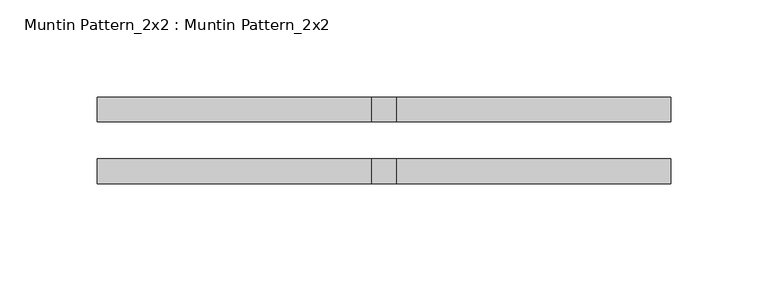
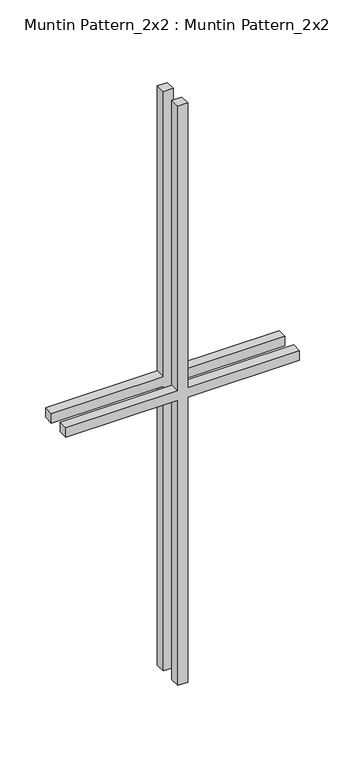
"""IFC4 building model written with IfcOpenShell, lengths in millimetres: proxy geometry, Muntin Pattern_2x2 : Muntin Pattern_2x2."""

from ifc_helpers import new_model, si_unit, frame, origin, place, context, project, spatial, polyline, outline, extrude, source, transform, mapped, element, save


def muntin_pattern_2x2_muntin_pattern_2x2_b3fe6957(model_context):
    return source(origin(), model_context, "Body", "SweptSolid", [
        extrude(outline(polyline([(393.7, -6.35), (393.7, -147.6375), (381.0, -147.6375), (381.0, -6.35), (0.0, -6.35), (0.0, 6.35), (381.0, 6.35), (381.0, 147.6375), (393.7, 147.6375), (393.7, 6.35), (774.7, 6.35), (774.7, -6.35), (393.7, -6.35)])), frame((0.0, 9.525, 0.0), z_axis=(0.0, 1.0, 0.0), x_axis=(0.0, 0.0, 1.0)), (0.0, 0.0, 1.0), 12.7),
        extrude(outline(polyline([(393.7, -6.35), (393.7, -147.6375), (381.0, -147.6375), (381.0, -6.35), (0.0, -6.35), (0.0, 6.35), (381.0, 6.35), (381.0, 147.6375), (393.7, 147.6375), (393.7, 6.35), (774.7, 6.35), (774.7, -6.35), (393.7, -6.35)])), frame((0.0, -22.225, 0.0), z_axis=(0.0, 1.0, 0.0), x_axis=(0.0, 0.0, 1.0)), (0.0, 0.0, 1.0), 12.7),
    ])


if __name__ == "__main__":
    model = new_model("IFC4")
    model_context = context("Model", 3, world=origin())
    ifc_project = project(units=[si_unit("LENGTHUNIT", "METRE", prefix="MILLI")], contexts=[model_context])
    site = spatial("IfcSite", under=ifc_project)
    building = spatial("IfcBuilding", under=site)
    placement = place(None, origin())
    muntin_pattern_2x2_muntin_pattern_2x2_shape = muntin_pattern_2x2_muntin_pattern_2x2_b3fe6957(model_context)
    element("IfcBuildingElementProxy", 1, Name="Muntin Pattern_2x2 : Muntin Pattern_2x2", ObjectType="Muntin Pattern_2x2 : Muntin Pattern_2x2", at=placement, inside=building, context=model_context, shape_type="MappedRepresentation", body=[
        mapped(muntin_pattern_2x2_muntin_pattern_2x2_shape, transform((0.0, 0.0, 0.0), x_axis=(1.0, 0.0, 0.0), y_axis=(0.0, 1.0, 0.0), z_axis=(0.0, 0.0, 1.0))),
    ])
    save(model, "model.ifc")

# Revit data of these elements
# Type "Muntin Pattern_2x2 : Muntin Pattern_2x2"
#   Width [instance default] = 4 ft
#   Thickness = 0.041667 ft
#   Height [instance default] = 4 ft
#   Distance = 0.0625 ft
#   Interior Material [instance default] = none
#   Exterior Material [instance default] = none
#   Default Elevation = 0
# Element 1 (IfcBuildingElementProxy, "Muntin Pattern_2x2 : Muntin Pattern_2x2")
#   Width = 0.96875 ft
#   Height = 2.541667 ft
#   Interior Material = Wood - Stained
#   Exterior Material = Clad - White
#   Materials on its faces: "Clad - White", "Wood - Stained"
# Materials
#   "Clad - White": class "Wood", colour RGB 242 242 238, transparency 0, Cost = 0
#   "Wood - Stained": class "Wood", colour RGB 224 178 126, transparency 0, Cost = 0
